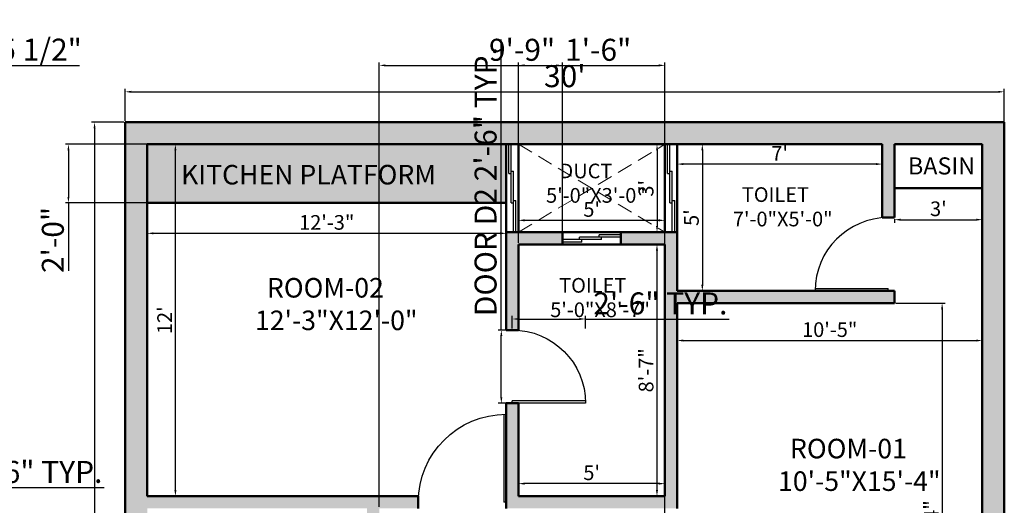
# Model space of a CAD drawing. Units: inches. Extents: x 3274 to 5176, y 1085 to 2172.
# Tile 16 of 16: x 4733 to 5136, y 1377 to 1575. Entities that reach past the tile are written whole.
import ezdxf

# ---------------------------------------------------------------- set-up
doc = ezdxf.new("R2010")
doc.units = ezdxf.units.IN
doc.linetypes.add('DASHED', pattern=[19.05, 12.7, -6.35])
for name, color, linetype, lineweight in [('A-ANNO-DIMS', 2, 'Continuous', 18), ('A-AREA-IDEN', 3, 'Continuous', 25), ('A-DOOR', 4, 'Continuous', 25), ('A-FLOR-OPEN', 7, 'DASHED', 18), ('A-FLOR-PATT', 252, 'Continuous', 13), ('A-GLAZ', 5, 'Continuous', 25), ('A-WALL', 7, 'Continuous', 50), ('A-WALL-PATT', 8, 'Continuous', 13)]:
    doc.layers.add(name, color=color, linetype=linetype, lineweight=lineweight)
doc.styles.get("Standard").update_dxf_attribs({"font": 'arial.ttf'})
doc.dimstyles.new('ISO-25', dxfattribs={"dimtxt": 9, "dimasz": 2.5, "dimexe": 1.25, "dimexo": 0.625, "dimtad": 1, "dimdec": 1, "dimlunit": 3, "dimtxsty": 'Standard', "dimcen": 2.5, "dimclrd": 4, "dimclre": 4, "dimclrt": 1, "dimadec": 0, "dimazin": 0, "dimtfac": 1, "dimtdec": 1, "dimtmove": 0, "dimatfit": 3, "dimfxl": 1, "dimarcsym": 0})

# ---------------------------------------------------------------- blocks, each defined once
blk = doc.blocks.new('*D4')
at = {"layer": 'A-ANNO-DIMS', "color": 0, "lineweight": -2, "transparency": 16777216}
for p, q in [((4775.78, 1533.98), (4775.78, 1547.09)), ((4778.28, 1545.84), (5133.28, 1545.84)), ((5135.78, 1533.98), (5135.78, 1547.09))]:
    blk.add_line(p, q, dxfattribs=at)
at = {"layer": 'A-ANNO-DIMS', "color": 0, "transparency": 16777216}
for points in [[(4778.28, 1546.26), (4778.28, 1545.43), (4775.78, 1545.84)], [(5133.28, 1546.26), (5133.28, 1545.43), (5135.78, 1545.84)]]:
    blk.add_solid(points, dxfattribs=at)
at = {"layer": 'Defpoints', "color": 0, "transparency": 16777216}
for p in [(5135.78, 1545.84), (4775.78, 1533.35), (5135.78, 1533.35)]:
    blk.add_point(p, dxfattribs=at)
at = {"layer": 'A-ANNO-DIMS', "color": 0, "transparency": 16777216, "insert": (4955.78, 1551.07), "char_height": 9, "attachment_point": 5}
blk.add_mtext("30'", dxfattribs=at)
blk = doc.blocks.new('*D5')
at = {"layer": 'A-ANNO-DIMS', "color": 0, "lineweight": -2, "transparency": 16777216}
for p, q in [((4775.16, 1533.35), (4761.93, 1533.35)), ((4763.18, 1530.85), (4763.18, 1175.85)), ((4775.16, 1173.35), (4761.93, 1173.35))]:
    blk.add_line(p, q, dxfattribs=at)
at = {"layer": 'A-ANNO-DIMS', "color": 0, "transparency": 16777216}
for points in [[(4762.76, 1530.85), (4763.6, 1530.85), (4763.18, 1533.35)], [(4762.76, 1175.85), (4763.6, 1175.85), (4763.18, 1173.35)]]:
    blk.add_solid(points, dxfattribs=at)
at = {"layer": 'Defpoints', "color": 0, "transparency": 16777216}
for p in [(4775.78, 1533.35), (4763.18, 1173.35), (4775.78, 1173.35)]:
    blk.add_point(p, dxfattribs=at)
at = {"layer": 'A-ANNO-DIMS', "color": 0, "transparency": 16777216, "insert": (4757.96, 1353.35), "char_height": 9, "attachment_point": 5, "rotation": 90}
blk.add_mtext("30'", dxfattribs=at)
blk = doc.blocks.new('1')
for p, q in [((0, 36), (0, 0)), ((1, 36), (1, 0)), ((0, 0), (1, 0))]:
    blk.add_line(p, q)
blk.add_arc((0, 0), 36, 0, 90)
blk = doc.blocks.new('2')
for p, q in [((0, 30), (0, 0)), ((1, 30), (1, 0)), ((0, 0), (1, 0))]:
    blk.add_line(p, q)
blk.add_arc((0, 0), 30, 0, 90)
blk = doc.blocks.new('*D93')
at = {"layer": 'A-ANNO-DIMS', "color": 0, "lineweight": -2, "transparency": 16777216}
for p, q in [((4785.41, 1524.35), (4797.55, 1524.35)), ((4796.3, 1382.85), (4796.3, 1521.85)), ((4785.41, 1380.35), (4797.55, 1380.35))]:
    blk.add_line(p, q, dxfattribs=at)
at = {"layer": 'A-ANNO-DIMS', "color": 0, "transparency": 16777216}
for points in [[(4795.88, 1521.85), (4796.71, 1521.85), (4796.3, 1524.35)], [(4795.88, 1382.85), (4796.71, 1382.85), (4796.3, 1380.35)]]:
    blk.add_solid(points, dxfattribs=at)
at = {"layer": 'Defpoints', "color": 0, "transparency": 16777216}
for p in [(4784.78, 1524.35), (4796.3, 1524.35), (4784.78, 1380.35)]:
    blk.add_point(p, dxfattribs=at)
at = {"layer": 'A-ANNO-DIMS', "color": 0, "transparency": 16777216, "insert": (4792.66, 1452.35), "char_height": 6, "attachment_point": 5, "rotation": 90}
blk.add_mtext("12'", dxfattribs=at)
blk = doc.blocks.new('*D94')
at = {"layer": 'A-ANNO-DIMS', "color": 0, "lineweight": -2, "transparency": 16777216}
for p, q in [((4784.78, 1499.73), (4784.78, 1486.67)), ((4931.78, 1499.73), (4931.78, 1486.67)), ((4787.28, 1487.92), (4929.28, 1487.92))]:
    blk.add_line(p, q, dxfattribs=at)
at = {"layer": 'A-ANNO-DIMS', "color": 0, "transparency": 16777216}
for points in [[(4787.28, 1488.34), (4787.28, 1487.5), (4784.78, 1487.92)], [(4929.28, 1488.34), (4929.28, 1487.5), (4931.78, 1487.92)]]:
    blk.add_solid(points, dxfattribs=at)
at = {"layer": 'Defpoints', "color": 0, "transparency": 16777216}
for p in [(4784.78, 1500.35), (4931.78, 1500.35), (4931.78, 1487.92)]:
    blk.add_point(p, dxfattribs=at)
at = {"layer": 'A-ANNO-DIMS', "color": 0, "transparency": 16777216, "insert": (4858.28, 1491.61), "char_height": 6, "attachment_point": 5}
blk.add_mtext('12\'-3"', dxfattribs=at)
blk = doc.blocks.new('*D95')
at = {"layer": 'A-ANNO-DIMS', "color": 0, "lineweight": -2, "transparency": 16777216}
for p, q in [((4996.16, 1483.35), (4992.29, 1483.35)), ((4993.54, 1480.85), (4993.54, 1382.85)), ((4996.16, 1380.35), (4992.29, 1380.35))]:
    blk.add_line(p, q, dxfattribs=at)
at = {"layer": 'A-ANNO-DIMS', "color": 0, "transparency": 16777216}
for points in [[(4993.12, 1480.85), (4993.95, 1480.85), (4993.54, 1483.35)], [(4993.12, 1382.85), (4993.95, 1382.85), (4993.54, 1380.35)]]:
    blk.add_solid(points, dxfattribs=at)
at = {"layer": 'Defpoints', "color": 0, "transparency": 16777216}
for p in [(4996.78, 1483.35), (4993.54, 1380.35), (4996.78, 1380.35)]:
    blk.add_point(p, dxfattribs=at)
at = {"layer": 'A-ANNO-DIMS', "color": 0, "transparency": 16777216, "insert": (4989.85, 1431.85), "char_height": 6, "attachment_point": 5, "rotation": 90}
blk.add_mtext('8\'-7"', dxfattribs=at)
blk = doc.blocks.new('*D96')
at = {"layer": 'A-ANNO-DIMS', "color": 0, "lineweight": -2, "transparency": 16777216}
for p, q in [((4936.78, 1380.98), (4936.78, 1386.71)), ((4994.28, 1385.46), (4939.28, 1385.46)), ((4996.78, 1380.98), (4996.78, 1386.71))]:
    blk.add_line(p, q, dxfattribs=at)
at = {"layer": 'A-ANNO-DIMS', "color": 0, "transparency": 16777216}
for points in [[(4939.28, 1385.88), (4939.28, 1385.05), (4936.78, 1385.46)], [(4994.28, 1385.88), (4994.28, 1385.05), (4996.78, 1385.46)]]:
    blk.add_solid(points, dxfattribs=at)
at = {"layer": 'Defpoints', "color": 0, "transparency": 16777216}
for p in [(4936.78, 1385.46), (4936.78, 1380.35), (4996.78, 1380.35)]:
    blk.add_point(p, dxfattribs=at)
at = {"layer": 'A-ANNO-DIMS', "color": 0, "transparency": 16777216, "insert": (4966.78, 1389.14), "char_height": 6, "attachment_point": 5}
blk.add_mtext("5'", dxfattribs=at)
blk = doc.blocks.new('*D97')
at = {"layer": 'A-ANNO-DIMS', "color": 0, "lineweight": -2, "transparency": 16777216}
for p, q in [((5001.78, 1458.73), (5001.78, 1442.79)), ((5126.78, 1458.73), (5126.78, 1442.79)), ((5004.28, 1444.04), (5124.28, 1444.04))]:
    blk.add_line(p, q, dxfattribs=at)
at = {"layer": 'A-ANNO-DIMS', "color": 0, "transparency": 16777216}
for points in [[(5004.28, 1444.46), (5004.28, 1443.62), (5001.78, 1444.04)], [(5124.28, 1444.46), (5124.28, 1443.62), (5126.78, 1444.04)]]:
    blk.add_solid(points, dxfattribs=at)
at = {"layer": 'Defpoints', "color": 0, "transparency": 16777216}
for p in [(5001.78, 1459.35), (5126.78, 1459.35), (5126.78, 1444.04)]:
    blk.add_point(p, dxfattribs=at)
at = {"layer": 'A-ANNO-DIMS', "color": 0, "transparency": 16777216, "insert": (5064.28, 1447.73), "char_height": 6, "attachment_point": 5}
blk.add_mtext('10\'-5"', dxfattribs=at)
blk = doc.blocks.new('*D98')
at = {"layer": 'A-ANNO-DIMS', "color": 0, "lineweight": -2, "transparency": 16777216}
for p, q in [((5091.41, 1459.35), (5111.56, 1459.35)), ((5110.31, 1456.85), (5110.31, 1277.85)), ((5091.41, 1275.35), (5111.56, 1275.35))]:
    blk.add_line(p, q, dxfattribs=at)
at = {"layer": 'A-ANNO-DIMS', "color": 0, "transparency": 16777216}
for points in [[(5109.9, 1456.85), (5110.73, 1456.85), (5110.31, 1459.35)], [(5109.9, 1277.85), (5110.73, 1277.85), (5110.31, 1275.35)]]:
    blk.add_solid(points, dxfattribs=at)
at = {"layer": 'Defpoints', "color": 0, "transparency": 16777216}
for p in [(5090.78, 1459.35), (5090.78, 1275.35), (5110.31, 1275.35)]:
    blk.add_point(p, dxfattribs=at)
at = {"layer": 'A-ANNO-DIMS', "color": 0, "transparency": 16777216, "insert": (5106.62, 1367.35), "char_height": 6, "attachment_point": 5, "rotation": 90}
blk.add_mtext('15\'-4"', dxfattribs=at)
blk = doc.blocks.new('*D99')
at = {"layer": 'A-ANNO-DIMS', "color": 0, "lineweight": -2, "transparency": 16777216}
for p, q in [((5002.41, 1524.35), (5013.36, 1524.35)), ((5012.11, 1521.85), (5012.11, 1466.85)), ((5002.41, 1464.35), (5013.36, 1464.35))]:
    blk.add_line(p, q, dxfattribs=at)
at = {"layer": 'A-ANNO-DIMS', "color": 0, "transparency": 16777216}
for points in [[(5011.69, 1521.85), (5012.52, 1521.85), (5012.11, 1524.35)], [(5011.69, 1466.85), (5012.52, 1466.85), (5012.11, 1464.35)]]:
    blk.add_solid(points, dxfattribs=at)
at = {"layer": 'Defpoints', "color": 0, "transparency": 16777216}
for p in [(5001.78, 1524.35), (5001.78, 1464.35), (5012.11, 1464.35)]:
    blk.add_point(p, dxfattribs=at)
at = {"layer": 'A-ANNO-DIMS', "color": 0, "transparency": 16777216, "insert": (5008.43, 1494.35), "char_height": 6, "attachment_point": 5, "rotation": 90}
blk.add_mtext("5'", dxfattribs=at)
blk = doc.blocks.new('*D100')
at = {"layer": 'A-ANNO-DIMS', "color": 0, "lineweight": -2, "transparency": 16777216}
for p, q in [((5001.78, 1523.73), (5001.78, 1515.01)), ((5085.78, 1523.73), (5085.78, 1515.01)), ((5083.28, 1516.26), (5004.28, 1516.26))]:
    blk.add_line(p, q, dxfattribs=at)
at = {"layer": 'A-ANNO-DIMS', "color": 0, "transparency": 16777216}
for points in [[(5004.28, 1516.67), (5004.28, 1515.84), (5001.78, 1516.26)], [(5083.28, 1516.67), (5083.28, 1515.84), (5085.78, 1516.26)]]:
    blk.add_solid(points, dxfattribs=at)
at = {"layer": 'Defpoints', "color": 0, "transparency": 16777216}
for p in [(5001.78, 1524.35), (5085.78, 1524.35), (5001.78, 1516.26)]:
    blk.add_point(p, dxfattribs=at)
at = {"layer": 'A-ANNO-DIMS', "color": 0, "transparency": 16777216, "insert": (5043.78, 1519.88), "char_height": 6, "attachment_point": 5}
blk.add_mtext("7'", dxfattribs=at)
blk = doc.blocks.new('*D101')
at = {"layer": 'A-ANNO-DIMS', "color": 0, "lineweight": -2, "transparency": 16777216}
for p, q in [((5090.78, 1493.73), (5090.78, 1492.25)), ((5093.28, 1493.5), (5124.28, 1493.5)), ((5126.78, 1493.73), (5126.78, 1492.25))]:
    blk.add_line(p, q, dxfattribs=at)
at = {"layer": 'A-ANNO-DIMS', "color": 0, "transparency": 16777216}
for points in [[(5093.28, 1493.92), (5093.28, 1493.09), (5090.78, 1493.5)], [(5124.28, 1493.92), (5124.28, 1493.09), (5126.78, 1493.5)]]:
    blk.add_solid(points, dxfattribs=at)
at = {"layer": 'Defpoints', "color": 0, "transparency": 16777216}
for p in [(5090.78, 1494.35), (5126.78, 1494.35), (5126.78, 1493.5)]:
    blk.add_point(p, dxfattribs=at)
at = {"layer": 'A-ANNO-DIMS', "color": 0, "transparency": 16777216, "insert": (5108.78, 1497.19), "char_height": 6, "attachment_point": 5}
blk.add_mtext("3'", dxfattribs=at)
blk = doc.blocks.new('*D102')
at = {"layer": 'A-ANNO-DIMS', "color": 0, "lineweight": -2, "transparency": 16777216}
for p, q in [((4996.16, 1524.35), (4992.3, 1524.35)), ((4993.55, 1521.85), (4993.55, 1490.85)), ((4996.16, 1488.35), (4992.3, 1488.35))]:
    blk.add_line(p, q, dxfattribs=at)
at = {"layer": 'A-ANNO-DIMS', "color": 0, "transparency": 16777216}
for points in [[(4993.14, 1521.85), (4993.97, 1521.85), (4993.55, 1524.35)], [(4993.14, 1490.85), (4993.97, 1490.85), (4993.55, 1488.35)]]:
    blk.add_solid(points, dxfattribs=at)
at = {"layer": 'Defpoints', "color": 0, "transparency": 16777216}
for p in [(4996.78, 1524.35), (4993.55, 1488.35), (4996.78, 1488.35)]:
    blk.add_point(p, dxfattribs=at)
at = {"layer": 'A-ANNO-DIMS', "color": 0, "transparency": 16777216, "insert": (4989.86, 1506.35), "char_height": 6, "attachment_point": 5, "rotation": 90}
blk.add_mtext("3'", dxfattribs=at)
blk = doc.blocks.new('*D103')
at = {"layer": 'A-ANNO-DIMS', "color": 0, "lineweight": -2, "transparency": 16777216}
for p, q in [((4936.78, 1488.98), (4936.78, 1494.48)), ((4994.28, 1493.23), (4939.28, 1493.23)), ((4996.78, 1488.98), (4996.78, 1494.48))]:
    blk.add_line(p, q, dxfattribs=at)
at = {"layer": 'A-ANNO-DIMS', "color": 0, "transparency": 16777216}
for points in [[(4939.28, 1493.65), (4939.28, 1492.81), (4936.78, 1493.23)], [(4994.28, 1493.65), (4994.28, 1492.81), (4996.78, 1493.23)]]:
    blk.add_solid(points, dxfattribs=at)
at = {"layer": 'Defpoints', "color": 0, "transparency": 16777216}
for p in [(4936.78, 1493.23), (4936.78, 1488.35), (4996.78, 1488.35)]:
    blk.add_point(p, dxfattribs=at)
at = {"layer": 'A-ANNO-DIMS', "color": 0, "transparency": 16777216, "insert": (4966.78, 1496.91), "char_height": 6, "attachment_point": 5}
blk.add_mtext("5'", dxfattribs=at)
blk = doc.blocks.new('WIN-24')
for p, q in [((4552.19, 1485.35), (4536.19, 1485.35)), ((4544.19, 1484.35), (4536.19, 1484.35)), ((4560.19, 1486.35), (4543.19, 1486.35)), ((4543.19, 1485.35), (4543.19, 1486.35)), ((4544.19, 1484.35), (4544.19, 1485.35)), ((4551.19, 1486.35), (4551.19, 1487.35)), ((4560.19, 1487.35), (4551.19, 1487.35)), ((4552.19, 1485.35), (4552.19, 1486.35))]:
    blk.add_line(p, q)
blk = doc.blocks.new('WIN-36')
for p, q in [((4514.19, 1512.35), (4514.19, 1524.35)), ((4515.19, 1500.35), (4515.19, 1524.35)), ((4514.19, 1512.35), (4515.19, 1512.35)), ((4515.19, 1513.35), (4516.19, 1513.35)), ((4516.19, 1488.35), (4516.19, 1513.35)), ((4515.19, 1500.35), (4516.19, 1500.35)), ((4516.19, 1501.35), (4517.19, 1501.35)), ((4517.19, 1488.35), (4517.19, 1501.35))]:
    blk.add_line(p, q)
blk = doc.blocks.new('*D116')
at = {"layer": 'A-ANNO-DIMS', "color": 4, "lineweight": -2, "transparency": 16777216}
for p, q in [((4929.78, 1448.35), (4929.78, 1567.29)), ((4933.66, 1448.35), (4928.53, 1448.35)), ((4929.78, 1420.85), (4929.78, 1445.85)), ((4933.66, 1418.35), (4928.53, 1418.35))]:
    blk.add_line(p, q, dxfattribs=at)
at = {"layer": 'A-ANNO-DIMS', "color": 4, "transparency": 16777216}
for points in [[(4929.37, 1445.85), (4930.2, 1445.85), (4929.78, 1448.35)], [(4929.37, 1420.85), (4930.2, 1420.85), (4929.78, 1418.35)]]:
    blk.add_solid(points, dxfattribs=at)
at = {"layer": 'Defpoints', "color": 0, "transparency": 16777216}
for p in [(4929.78, 1448.35), (4934.28, 1448.35), (4934.28, 1418.35)]:
    blk.add_point(p, dxfattribs=at)
at = {"layer": 'A-ANNO-DIMS', "color": 1, "transparency": 16777216, "insert": (4924.5, 1509.07), "char_height": 9, "attachment_point": 5, "rotation": 90}
blk.add_mtext('DOOR D2 2\'-6" TYP.', dxfattribs=at)
blk = doc.blocks.new('*D117')
at = {"layer": 'A-ANNO-DIMS', "color": 4, "lineweight": -2, "transparency": 16777216}
for p, q in [((4934.28, 1448.98), (4934.28, 1454.1)), ((4936.78, 1452.85), (4961.78, 1452.85)), ((4964.28, 1448.98), (4964.28, 1454.1)), ((4964.28, 1452.85), (5023.05, 1452.85))]:
    blk.add_line(p, q, dxfattribs=at)
at = {"layer": 'A-ANNO-DIMS', "color": 4, "transparency": 16777216}
for points in [[(4936.78, 1453.27), (4936.78, 1452.44), (4934.28, 1452.85)], [(4961.78, 1453.27), (4961.78, 1452.44), (4964.28, 1452.85)]]:
    blk.add_solid(points, dxfattribs=at)
at = {"layer": 'Defpoints', "color": 0, "transparency": 16777216}
for p in [(4964.28, 1452.85), (4934.28, 1448.35), (4964.28, 1448.35)]:
    blk.add_point(p, dxfattribs=at)
at = {"layer": 'A-ANNO-DIMS', "color": 1, "transparency": 16777216, "insert": (4994.91, 1458.07), "char_height": 9, "attachment_point": 5}
blk.add_mtext('2\'-6" TYP.', dxfattribs=at)
blk = doc.blocks.new('*D137')
at = {"layer": 'A-ANNO-DIMS', "color": 4, "lineweight": -2, "transparency": 16777216}
for p, q in [((4654.05, 1370.36), (4654.05, 1385.14)), ((4656.55, 1383.89), (4705.7, 1383.89)), ((4708.2, 1370.36), (4708.2, 1385.14)), ((4708.2, 1383.89), (4767.17, 1383.89))]:
    blk.add_line(p, q, dxfattribs=at)
at = {"layer": 'A-ANNO-DIMS', "color": 4, "transparency": 16777216}
for points in [[(4656.55, 1384.31), (4656.55, 1383.47), (4654.05, 1383.89)], [(4705.7, 1384.31), (4705.7, 1383.47), (4708.2, 1383.89)]]:
    blk.add_solid(points, dxfattribs=at)
at = {"layer": 'Defpoints', "color": 0, "transparency": 16777216}
for p in [(4708.2, 1383.89), (4654.05, 1369.73), (4708.2, 1369.73)]:
    blk.add_point(p, dxfattribs=at)
at = {"layer": 'A-ANNO-DIMS', "color": 1, "transparency": 16777216, "insert": (4738.94, 1389.11), "char_height": 9, "attachment_point": 5}
blk.add_mtext('4\'-6" TYP.', dxfattribs=at)
blk = doc.blocks.new('*D157')
at = {"layer": 'A-ANNO-DIMS', "color": 4, "lineweight": -2, "transparency": 16777216}
for p, q in [((4678.86, 1444.32), (4678.86, 1557.9)), ((4681.36, 1556.65), (4705.69, 1556.65)), ((4708.19, 1380.98), (4708.19, 1557.9)), ((4708.19, 1556.65), (4756.99, 1556.65))]:
    blk.add_line(p, q, dxfattribs=at)
at = {"layer": 'A-ANNO-DIMS', "color": 4, "transparency": 16777216}
for points in [[(4681.36, 1557.07), (4681.36, 1556.24), (4678.86, 1556.65)], [(4705.69, 1557.07), (4705.69, 1556.24), (4708.19, 1556.65)]]:
    blk.add_solid(points, dxfattribs=at)
at = {"layer": 'Defpoints', "color": 0, "transparency": 16777216}
for p in [(4708.19, 1556.65), (4678.86, 1443.7), (4708.19, 1380.35)]:
    blk.add_point(p, dxfattribs=at)
at = {"layer": 'A-ANNO-DIMS', "color": 1, "transparency": 16777216, "insert": (4733.84, 1561.93), "char_height": 9, "attachment_point": 5}
blk.add_mtext('2\'-5 1/2"', dxfattribs=at)
blk = doc.blocks.new('*D184')
at = {"layer": 'A-ANNO-DIMS', "color": 4, "lineweight": -2, "transparency": 16777216}
for p, q in [((4931.16, 1524.35), (4751.23, 1524.35)), ((4752.48, 1521.85), (4752.48, 1502.85)), ((4931.16, 1500.35), (4751.23, 1500.35)), ((4752.48, 1500.35), (4752.48, 1472.53))]:
    blk.add_line(p, q, dxfattribs=at)
at = {"layer": 'A-ANNO-DIMS', "color": 4, "transparency": 16777216}
for points in [[(4752.07, 1521.85), (4752.9, 1521.85), (4752.48, 1524.35)], [(4752.07, 1502.85), (4752.9, 1502.85), (4752.48, 1500.35)]]:
    blk.add_solid(points, dxfattribs=at)
at = {"layer": 'Defpoints', "color": 0, "transparency": 16777216}
for p in [(4931.78, 1524.35), (4752.48, 1500.35), (4931.78, 1500.35)]:
    blk.add_point(p, dxfattribs=at)
at = {"layer": 'A-ANNO-DIMS', "color": 1, "transparency": 16777216, "insert": (4747.26, 1485.19), "char_height": 9, "attachment_point": 5, "rotation": 90}
blk.add_mtext('2\'-0"', dxfattribs=at)
blk = doc.blocks.new('*D188')
at = {"layer": 'A-ANNO-DIMS', "color": 4, "lineweight": -2, "transparency": 16777216}
for p, q in [((4879.78, 1375.98), (4879.78, 1557.9)), ((4882.28, 1556.65), (4994.28, 1556.65)), ((4996.78, 1339.98), (4996.78, 1557.9))]:
    blk.add_line(p, q, dxfattribs=at)
at = {"layer": 'A-ANNO-DIMS', "color": 4, "transparency": 16777216}
for points in [[(4882.28, 1557.07), (4882.28, 1556.24), (4879.78, 1556.65)], [(4994.28, 1557.07), (4994.28, 1556.24), (4996.78, 1556.65)]]:
    blk.add_solid(points, dxfattribs=at)
at = {"layer": 'Defpoints', "color": 0, "transparency": 16777216}
for p in [(4996.78, 1556.65), (4879.78, 1375.35), (4996.78, 1339.35)]:
    blk.add_point(p, dxfattribs=at)
at = {"layer": 'A-ANNO-DIMS', "color": 1, "transparency": 16777216, "insert": (4938.28, 1561.87), "char_height": 9, "attachment_point": 5}
blk.add_mtext('9\'-9"', dxfattribs=at)
blk = doc.blocks.new('*D191')
at = {"layer": 'A-ANNO-DIMS', "color": 4, "lineweight": -2, "transparency": 16777216}
for p, q in [((4936.78, 1483.98), (4936.78, 1557.9)), ((4939.28, 1556.65), (4952.28, 1556.65)), ((4954.78, 1483.98), (4954.78, 1557.9)), ((4954.78, 1556.65), (4981.61, 1556.65))]:
    blk.add_line(p, q, dxfattribs=at)
at = {"layer": 'A-ANNO-DIMS', "color": 4, "transparency": 16777216}
for points in [[(4939.28, 1557.07), (4939.28, 1556.24), (4936.78, 1556.65)], [(4952.28, 1557.07), (4952.28, 1556.24), (4954.78, 1556.65)]]:
    blk.add_solid(points, dxfattribs=at)
at = {"layer": 'Defpoints', "color": 0, "transparency": 16777216}
for p in [(4954.78, 1556.65), (4936.78, 1483.35), (4954.78, 1483.35)]:
    blk.add_point(p, dxfattribs=at)
at = {"layer": 'A-ANNO-DIMS', "color": 1, "transparency": 16777216, "insert": (4969.45, 1561.87), "char_height": 9, "attachment_point": 5}
blk.add_mtext('1\'-6"', dxfattribs=at)

msp = doc.modelspace()

# ---------------------------------------------------------------- hatches: boundary and pattern name
at = {"layer": 'A-FLOR-PATT'}
h = msp.add_hatch(color=256, dxfattribs=at)
h.dxf.hatch_style = 1
h.paths.add_polyline_path([(4931.78, 1500.35), (4931.78, 1524.35), (4784.78, 1524.35), (4784.78, 1500.35)])
h.paths.add_polyline_path([(4795.81, 1503.41), (4912.82, 1503.41), (4912.82, 1519.9), (4795.81, 1519.9)], flags=24)
at = {"layer": 'A-WALL-PATT'}
h = msp.add_hatch(color=256, dxfattribs=at)
h.dxf.hatch_style = 1
h.paths.add_polyline_path([(4819.78, 1319.35), (4819.78, 1339.35), (4814.78, 1339.35), (4814.78, 1314.35), (4844.78, 1314.35), (4844.78, 1319.35)], flags=17)
h.paths.add_polyline_path([(4775.78, 1173.35), (4808.78, 1173.35), (4808.78, 1182.35), (4784.78, 1182.35), (4784.78, 1375.35), (4874.78, 1375.35), (4874.78, 1314.35), (4895.78, 1314.35), (4895.78, 1319.35), (4879.78, 1319.35), (4879.78, 1375.35), (4895.78, 1375.35), (4895.78, 1380.35), (4784.78, 1380.35), (4784.78, 1524.35), (5085.78, 1524.35), (5085.78, 1494.35), (5090.78, 1494.35), (5090.78, 1524.35), (5126.78, 1524.35), (5126.78, 1275.35), (5094.28, 1275.35), (5094.28, 1266.35), (5126.78, 1266.35), (5126.78, 1182.35), (5084.78, 1182.35), (5084.78, 1173.35), (5135.78, 1173.35), (5135.78, 1533.35), (4775.78, 1533.35)])
h.paths.add_polyline_path([(4996.78, 1380.35), (4936.78, 1380.35), (4936.78, 1418.35), (4934.28, 1418.35), (4931.78, 1418.35), (4931.78, 1375.35), (5001.78, 1375.35), (5001.78, 1459.35), (5090.78, 1459.35), (5090.78, 1464.35), (5001.78, 1464.35), (5001.78, 1488.35), (4978.78, 1488.35), (4978.78, 1483.35), (4996.78, 1483.35)], flags=17)
h.paths.add_polyline_path([(4931.78, 1488.35), (4931.78, 1448.35), (4936.78, 1448.35), (4936.78, 1483.35), (4954.78, 1483.35), (4954.78, 1488.35)], flags=17)
h.paths.add_polyline_path([(5034.28, 1266.35), (5034.28, 1275.35), (5001.78, 1275.35), (5001.78, 1339.35), (4996.78, 1339.35), (4996.78, 1275.35), (4989.78, 1275.35), (4989.78, 1270.85), (4989.78, 1266.35)], flags=17)
h.paths.add_polyline_path([(4936.78, 1266.35), (4941.78, 1266.35), (4941.78, 1275.35), (4936.78, 1275.35), (4936.78, 1319.35), (4931.78, 1319.35), (4931.78, 1182.35), (4880.78, 1182.35), (4880.78, 1173.35), (4936.78, 1173.35)], flags=17)
h.paths.add_polyline_path([(4996.78, 1182.35), (4996.78, 1173.35), (5012.78, 1173.35), (5012.78, 1182.35)], flags=17)

# ---------------------------------------------------------------- linework, layer by layer
at = {"layer": 'A-FLOR-OPEN', "ltscale": 0.5}
for p, q in [((4936.78, 1524.35), (4996.78, 1488.35)), ((4936.78, 1488.35), (4996.78, 1524.35))]:
    msp.add_line(p, q, dxfattribs=at)
at = {"layer": 'A-WALL'}
for p, q in [((4784.78, 1524.35), (5085.78, 1524.35)), ((4784.78, 1380.35), (4784.78, 1524.35)), ((4931.78, 1448.35), (4931.78, 1524.35)), ((4936.78, 1488.35), (4936.78, 1524.35)), ((4996.78, 1524.35), (4996.78, 1488.35)), ((5001.78, 1524.35), (5001.78, 1464.35)), ((5085.78, 1524.35), (5085.78, 1494.35)), ((5090.78, 1524.35), (5090.78, 1494.35)), ((5090.78, 1524.35), (5126.78, 1524.35)), ((5126.78, 1524.35), (5126.78, 1275.35)), ((5090.78, 1506.35), (5126.78, 1506.35)), ((4784.78, 1500.35), (4931.78, 1500.35)), ((5085.78, 1494.35), (5090.78, 1494.35)), ((4931.78, 1488.35), (5001.78, 1488.35)), ((4954.78, 1483.35), (4954.78, 1488.35)), ((4978.78, 1483.35), (4978.78, 1488.35)), ((4936.78, 1483.35), (4996.78, 1483.35)), ((4936.78, 1448.35), (4936.78, 1483.35)), ((4996.78, 1483.35), (4996.78, 1380.35)), ((5001.78, 1464.35), (5090.78, 1464.35)), ((5090.78, 1464.35), (5090.78, 1459.35)), ((5001.78, 1459.35), (5090.78, 1459.35)), ((5001.78, 1459.35), (5001.78, 1375.35)), ((4931.78, 1448.35), (4936.78, 1448.35)), ((4931.78, 1375.35), (4931.78, 1418.35)), ((4931.78, 1418.35), (4936.78, 1418.35)), ((4936.78, 1380.35), (4936.78, 1418.35)), ((4784.78, 1380.35), (4895.78, 1380.35)), ((4895.78, 1375.35), (4895.78, 1380.35)), ((4936.78, 1380.35), (4996.78, 1380.35))]:
    msp.add_line(p, q, dxfattribs=at)
msp.add_lwpolyline([(4936.78, 1173.35), (4775.78, 1173.35), (4775.78, 1533.35), (5135.78, 1533.35), (5135.78, 1173.35), (4936.78, 1173.35)], dxfattribs=at)

# ---------------------------------------------------------------- block references
at = {"layer": 'A-DOOR', "rotation": 89.99999999999999}
msp.add_blockref('2', (5088.28, 1464.35), dxfattribs=at)
at = {"layer": 'A-DOOR', "xscale": -1, "rotation": 270}
msp.add_blockref('2', (4934.28, 1418.35), dxfattribs=at)
at = {"layer": 'A-DOOR', "xscale": -1}
msp.add_blockref('1', (4931.78, 1377.85), dxfattribs=at)
at = {"layer": 'A-GLAZ'}
for name, p in [('WIN-36', (418.6, 0)), ('WIN-36', (483.6, 0)), ('WIN-24', (418.6, 0))]:
    msp.add_blockref(name, p, dxfattribs=at)

# ---------------------------------------------------------------- texts
at = {"layer": 'A-AREA-IDEN', "attachment_point": 1}
for s, width, heights, insert, char_height in [('   DUCT\\P5\'-0"X3\'-0"', 58.0121, [16.24], (4948.11, 1516.44), 6), ('BASIN', 147.1149, [0], (5096.33, 1519.01), 7), ('KITCHEN PLATFORM', 147.1149, [0], (4798.63, 1515.92), 8), ('  TOILET\\P7\'-0"X5\'-0"', 58.0121, [16.24], (5024.61, 1506.77), 6), ('  ROOM-02\\P12\'-3"X12\'-0"', 58.0121, [0], (4828.89, 1469.63), 8), ('  TOILET\\P5\'-0"X8\'-7"', 58.0121, [16.24], (4949.8, 1469.63), 6), ('  ROOM-01\\P10\'-5"X15\'-4"', 58.0121, [0], (5043.11, 1403.82), 8)]:
    msp.add_mtext_dynamic_manual_height_columns(s, width=width, gutter_width=30, heights=heights, dxfattribs=dict(at, insert=insert, char_height=char_height))

# ---------------------------------------------------------------- dimensions: what is measured, and where the dimension line sits
at = {"layer": 'A-ANNO-DIMS'}
for base, p1, p2, override, picture, middle in [((4708.19, 1556.65), (4678.86, 1443.7), (4708.19, 1380.35), {"dimdec": 1, "dimlfac": 1, "dimrnd": 0, "dimzin": 1, "dimdsep": 46, "dimlunit": 4, "dimfrac": 2}, '*D157', (4733.84, 1561.93)), ((4996.78, 1556.65), (4879.78, 1375.35), (4996.78, 1339.35), {"dimdec": 1, "dimlfac": 1, "dimrnd": 0, "dimzin": 1, "dimdsep": 46, "dimlunit": 4, "dimfrac": 2}, '*D188', (4938.28, 1561.87)), ((4954.78, 1556.65), (4936.78, 1483.35), (4954.78, 1483.35), {"dimdec": 1, "dimlfac": 1, "dimrnd": 0, "dimzin": 1, "dimdsep": 46, "dimlunit": 4, "dimfrac": 2}, '*D191', (4969.45, 1561.87)), ((5135.78, 1545.84), (4775.78, 1533.35), (5135.78, 1533.35), {"dimclrd": 0, "dimclre": 0, "dimclrt": 0}, '*D4', (4955.78, 1551.07)), ((5001.78, 1516.26), (5085.78, 1524.35), (5001.78, 1524.35), {"dimtxt": 6, "dimclrd": 0, "dimclre": 0, "dimclrt": 0}, '*D100', (5043.78, 1519.88)), ((4931.78, 1487.92), (4784.78, 1500.35), (4931.78, 1500.35), {"dimtxt": 6, "dimclrd": 0, "dimclre": 0, "dimclrt": 0}, '*D94', (4858.28, 1491.61)), ((4936.78, 1493.23), (4996.78, 1488.35), (4936.78, 1488.35), {"dimtxt": 6, "dimclrd": 0, "dimclre": 0, "dimclrt": 0}, '*D103', (4966.78, 1496.91)), ((5126.78, 1493.5), (5090.78, 1494.35), (5126.78, 1494.35), {"dimtxt": 6, "dimclrd": 0, "dimclre": 0, "dimclrt": 0}, '*D101', (5108.78, 1497.19)), ((5126.78, 1444.04), (5001.78, 1459.35), (5126.78, 1459.35), {"dimtxt": 6, "dimclrd": 0, "dimclre": 0, "dimclrt": 0}, '*D97', (5064.28, 1447.73)), ((4936.78, 1385.46), (4996.78, 1380.35), (4936.78, 1380.35), {"dimtxt": 6, "dimclrd": 0, "dimclre": 0, "dimclrt": 0}, '*D96', (4966.78, 1389.14))]:
    dim = msp.add_linear_dim(base=base, p1=p1, p2=p2, dimstyle='ISO-25', override=override, dxfattribs=at)
    dim.commit()
    dim.dimension.update_dxf_attribs({"geometry": picture, "text_midpoint": middle})
dim = msp.add_linear_dim(base=(4929.78, 1448.35), p1=(4934.28, 1418.35), p2=(4934.28, 1448.35), angle=90, text='DOOR D2 <> TYP.', dimstyle='ISO-25', override={"dimdec": 1, "dimrnd": 0, "dimzin": 1, "dimlunit": 4, "dimfrac": 2}, dxfattribs=at)
dim.commit()
dim.dimension.update_dxf_attribs({"geometry": '*D116', "text_midpoint": (4924.5, 1509.07)})
for base, p1, p2, override, picture, middle in [((4763.18, 1173.35), (4775.78, 1533.35), (4775.78, 1173.35), {"dimclrd": 0, "dimclre": 0, "dimclrt": 0}, '*D5', (4757.96, 1353.35)), ((4752.48, 1500.35), (4931.78, 1524.35), (4931.78, 1500.35), {"dimdec": 1, "dimlfac": 1, "dimrnd": 0, "dimzin": 1, "dimdsep": 46, "dimlunit": 4, "dimfrac": 2}, '*D184', (4747.26, 1485.19)), ((4796.3, 1524.35), (4784.78, 1380.35), (4784.78, 1524.35), {"dimtxt": 6, "dimclrd": 0, "dimclre": 0, "dimclrt": 0}, '*D93', (4792.66, 1452.35)), ((4993.55, 1488.35), (4996.78, 1524.35), (4996.78, 1488.35), {"dimtxt": 6, "dimclrd": 0, "dimclre": 0, "dimclrt": 0}, '*D102', (4989.86, 1506.35)), ((5012.11, 1464.35), (5001.78, 1524.35), (5001.78, 1464.35), {"dimtxt": 6, "dimclrd": 0, "dimclre": 0, "dimclrt": 0}, '*D99', (5008.43, 1494.35)), ((4993.54, 1380.35), (4996.78, 1483.35), (4996.78, 1380.35), {"dimtxt": 6, "dimclrd": 0, "dimclre": 0, "dimclrt": 0}, '*D95', (4989.85, 1431.85)), ((5110.31, 1275.35), (5090.78, 1459.35), (5090.78, 1275.35), {"dimtxt": 6, "dimclrd": 0, "dimclre": 0, "dimclrt": 0}, '*D98', (5106.62, 1367.35))]:
    dim = msp.add_linear_dim(base=base, p1=p1, p2=p2, angle=90, dimstyle='ISO-25', override=override, dxfattribs=at)
    dim.commit()
    dim.dimension.update_dxf_attribs({"geometry": picture, "text_midpoint": middle})
for base, p1, p2, picture, middle in [((4964.28, 1452.85), (4934.28, 1448.35), (4964.28, 1448.35), '*D117', (4994.91, 1458.07)), ((4708.2003, 1383.8897), (4654.047, 1369.7311), (4708.2003, 1369.7311), '*D137', (4738.9362, 1389.1098))]:
    dim = msp.add_linear_dim(base=base, p1=p1, p2=p2, text='<> TYP.', dimstyle='ISO-25', override={"dimdec": 1, "dimrnd": 0, "dimzin": 1, "dimlunit": 4, "dimfrac": 2}, dxfattribs=at)
    dim.commit()
    dim.dimension.update_dxf_attribs({"geometry": picture, "text_midpoint": middle})

doc.saveas('drawing.dxf')
